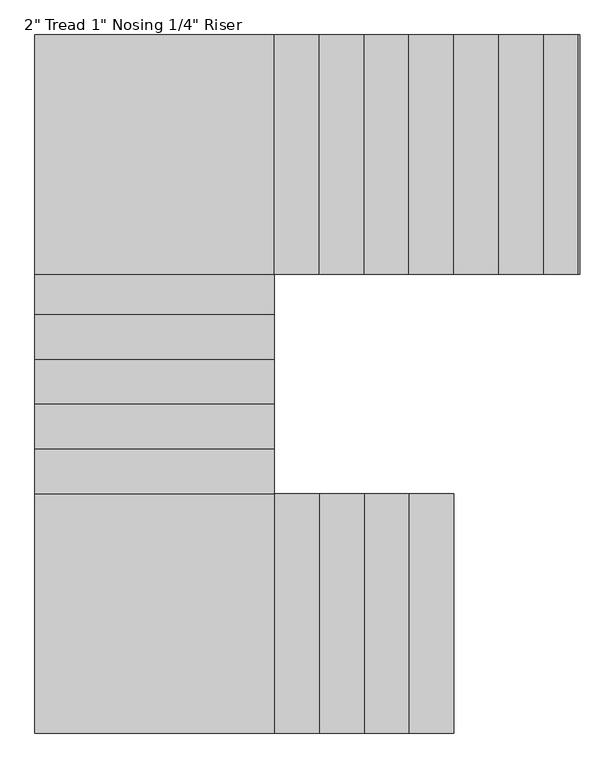
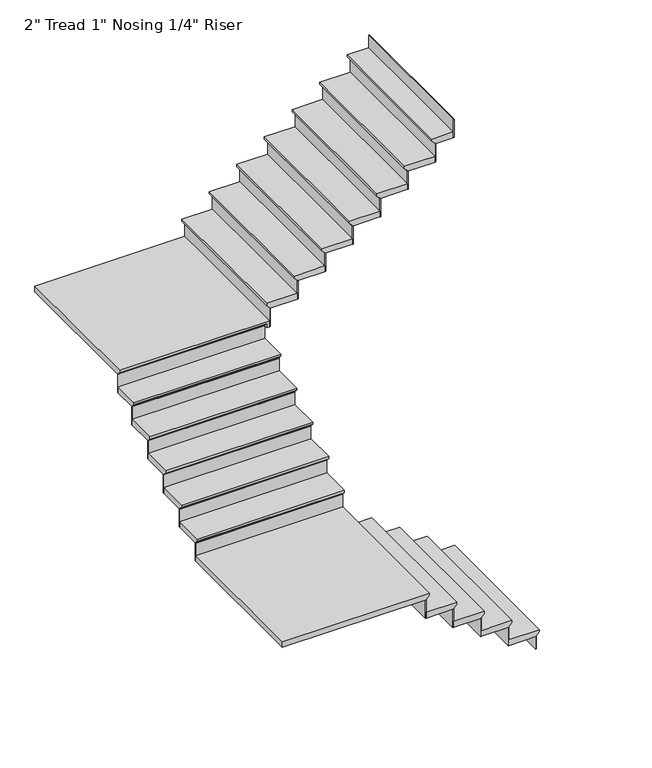
"""IFC4 building model written with IfcOpenShell, lengths in millimetres: stair flight geometry."""

from ifc_helpers import new_model, si_unit, origin, place, context, project, spatial, faceted_brep, source, transform, mapped, element, save


def stair_flight_abd4a925(model_context):
    return source(origin(), model_context, "Body", "Brep", [
        faceted_brep([(-2683.1105391, -1521.8373761, 9590.1710526), (-2683.1105391, -1521.8373761, 9609.2210526), (-2683.1105391, -2741.0373761, 9609.2210526), (-2683.1105391, -2741.0373761, 9590.1710526), (-2708.5105391, -1521.8373761, 9564.7710526), (-2708.5105391, -2741.0373761, 9564.7710526), (-2937.1105391, -1521.8373761, 9609.2210526), (-2937.1105391, -2741.0373761, 9609.2210526), (-2708.5105391, -2741.0373761, 9558.4210526), (-2937.1105391, -2741.0373761, 9558.4210526), (-2937.1105391, -1521.8373761, 9558.4210526), (-2708.5105391, -1521.8373761, 9558.4210526)], [[[0, 1, 2, 3]], [[4, 0, 3, 5]], [[2, 1, 6, 7]], [[8, 9, 10, 11]], [[2, 7, 9, 8, 5, 3]], [[8, 11, 4, 5]], [[6, 1, 0, 4, 11, 10]], [[7, 6, 10, 9]]]),
        faceted_brep([(-2708.5105391, -1521.8373761, 9558.4210526), (-2708.5105391, -1521.8373761, 9448.8), (-2714.8605391, -1521.8373761, 9448.8), (-2714.8605391, -1521.8373761, 9558.4210526), (-2708.5105391, -2741.0373761, 9558.4210526), (-2714.8605391, -2741.0373761, 9558.4210526), (-2714.8605391, -2741.0373761, 9448.8), (-2708.5105391, -2741.0373761, 9448.8)], [[[0, 1, 2, 3]], [[4, 5, 6, 7]], [[1, 0, 4, 7]], [[2, 1, 7, 6]], [[3, 2, 6, 5]], [[0, 3, 5, 4]]]),
        faceted_brep([(-2937.1105391, -1521.8373761, 9718.8421053), (-2937.1105391, -1521.8373761, 9558.4210526), (-2943.4605391, -1521.8373761, 9558.4210526), (-2943.4605391, -1521.8373761, 9718.8421053), (-2937.1105391, -2741.0373761, 9718.8421053), (-2943.4605391, -2741.0373761, 9718.8421053), (-2943.4605391, -2741.0373761, 9558.4210526), (-2937.1105391, -2741.0373761, 9558.4210526)], [[[0, 1, 2, 3]], [[4, 5, 6, 7]], [[1, 0, 4, 7]], [[2, 1, 7, 6]], [[3, 2, 6, 5]], [[0, 3, 5, 4]]]),
        faceted_brep([(-2911.7105391, -2741.0373761, 9769.6421053), (-2911.7105391, -1521.8373761, 9769.6421053), (-3165.7105391, -1521.8373761, 9769.6421053), (-3165.7105391, -2741.0373761, 9769.6421053), (-2937.1105391, -2741.0373761, 9718.8421053), (-3165.7105391, -2741.0373761, 9718.8421053), (-3165.7105391, -1521.8373761, 9718.8421053), (-2937.1105391, -1521.8373761, 9718.8421053), (-2937.1105391, -2741.0373761, 9725.1921053), (-2911.7105391, -2741.0373761, 9750.5921053), (-2937.1105391, -1521.8373761, 9725.1921053), (-2911.7105391, -1521.8373761, 9750.5921053)], [[[0, 1, 2, 3]], [[4, 5, 6, 7]], [[0, 3, 5, 4, 8, 9]], [[4, 7, 10, 8]], [[2, 1, 11, 10, 7, 6]], [[3, 2, 6, 5]], [[11, 1, 0, 9]], [[10, 11, 9, 8]]]),
        faceted_brep([(-3165.7105391, -1521.8373761, 9879.2631579), (-3165.7105391, -1521.8373761, 9718.8421053), (-3172.0605391, -1521.8373761, 9718.8421053), (-3172.0605391, -1521.8373761, 9879.2631579), (-3165.7105391, -2741.0373761, 9879.2631579), (-3172.0605391, -2741.0373761, 9879.2631579), (-3172.0605391, -2741.0373761, 9718.8421053), (-3165.7105391, -2741.0373761, 9718.8421053)], [[[0, 1, 2, 3]], [[4, 5, 6, 7]], [[1, 0, 4, 7]], [[2, 1, 7, 6]], [[3, 2, 6, 5]], [[0, 3, 5, 4]]]),
        faceted_brep([(-3140.3105391, -2741.0373761, 9930.0631579), (-3140.3105391, -1521.8373761, 9930.0631579), (-3394.3105391, -1521.8373761, 9930.0631579), (-3394.3105391, -2741.0373761, 9930.0631579), (-3165.7105391, -2741.0373761, 9879.2631579), (-3394.3105391, -2741.0373761, 9879.2631579), (-3394.3105391, -1521.8373761, 9879.2631579), (-3165.7105391, -1521.8373761, 9879.2631579), (-3165.7105391, -2741.0373761, 9885.6131579), (-3140.3105391, -2741.0373761, 9911.0131579), (-3165.7105391, -1521.8373761, 9885.6131579), (-3140.3105391, -1521.8373761, 9911.0131579)], [[[0, 1, 2, 3]], [[4, 5, 6, 7]], [[0, 3, 5, 4, 8, 9]], [[4, 7, 10, 8]], [[2, 1, 11, 10, 7, 6]], [[3, 2, 6, 5]], [[11, 1, 0, 9]], [[10, 11, 9, 8]]]),
        faceted_brep([(-3394.3105391, -1521.8373761, 10039.6842105), (-3394.3105391, -1521.8373761, 9879.2631579), (-3400.6605391, -1521.8373761, 9879.2631579), (-3400.6605391, -1521.8373761, 10039.6842105), (-3394.3105391, -2741.0373761, 10039.6842105), (-3400.6605391, -2741.0373761, 10039.6842105), (-3400.6605391, -2741.0373761, 9879.2631579), (-3394.3105391, -2741.0373761, 9879.2631579)], [[[0, 1, 2, 3]], [[4, 5, 6, 7]], [[1, 0, 4, 7]], [[2, 1, 7, 6]], [[3, 2, 6, 5]], [[0, 3, 5, 4]]]),
        faceted_brep([(-3368.9105391, -2741.0373761, 10090.4842105), (-3368.9105391, -1521.8373761, 10090.4842105), (-3622.9105391, -1521.8373761, 10090.4842105), (-3622.9105391, -2741.0373761, 10090.4842105), (-3394.3105391, -2741.0373761, 10039.6842105), (-3622.9105391, -2741.0373761, 10039.6842105), (-3622.9105391, -1521.8373761, 10039.6842105), (-3394.3105391, -1521.8373761, 10039.6842105), (-3394.3105391, -2741.0373761, 10046.0342105), (-3368.9105391, -2741.0373761, 10071.4342105), (-3394.3105391, -1521.8373761, 10046.0342105), (-3368.9105391, -1521.8373761, 10071.4342105)], [[[0, 1, 2, 3]], [[4, 5, 6, 7]], [[0, 3, 5, 4, 8, 9]], [[4, 7, 10, 8]], [[2, 1, 11, 10, 7, 6]], [[3, 2, 6, 5]], [[11, 1, 0, 9]], [[10, 11, 9, 8]]]),
        faceted_brep([(-3622.9105391, -1521.8373761, 10200.1052632), (-3622.9105391, -1521.8373761, 10039.6842105), (-3629.2605391, -1521.8373761, 10039.6842105), (-3629.2605391, -1521.8373761, 10200.1052632), (-3622.9105391, -2741.0373761, 10200.1052632), (-3629.2605391, -2741.0373761, 10200.1052632), (-3629.2605391, -2741.0373761, 10039.6842105), (-3622.9105391, -2741.0373761, 10039.6842105)], [[[0, 1, 2, 3]], [[4, 5, 6, 7]], [[1, 0, 4, 7]], [[2, 1, 7, 6]], [[3, 2, 6, 5]], [[0, 3, 5, 4]]]),
        faceted_brep([(-4816.7105391, -1496.4373761, 10250.9052632), (-4816.7105391, -2741.0373761, 10250.9052632), (-3597.5105391, -2741.0373761, 10250.9052632), (-3597.5105391, -1496.4373761, 10250.9052632), (-4816.7105391, -2741.0373761, 10200.1052632), (-4816.7105391, -1496.4373761, 10200.1052632), (-3597.5105391, -1496.4373761, 10200.1052632), (-3597.5105391, -1521.8373761, 10200.1052632), (-3622.9105391, -1521.8373761, 10200.1052632), (-3622.9105391, -2741.0373761, 10200.1052632), (-3622.9105391, -2741.0373761, 10206.4552632), (-3597.5105391, -2741.0373761, 10231.8552632), (-3622.9105391, -1521.8373761, 10206.4552632), (-3597.5105391, -1521.8373761, 10231.8552632)], [[[0, 1, 2, 3]], [[4, 5, 6, 7, 8, 9]], [[1, 0, 5, 4]], [[2, 1, 4, 9, 10, 11]], [[9, 8, 12, 10]], [[8, 7, 13, 12]], [[3, 2, 11, 13, 7, 6]], [[0, 3, 6, 5]], [[11, 10, 12, 13]]]),
        faceted_brep([(-3597.5105391, -1496.4373761, 10360.5263158), (-3597.5105391, -1496.4373761, 10200.1052632), (-3597.5105391, -1490.0873761, 10200.1052632), (-3597.5105391, -1490.0873761, 10360.5263158), (-4816.7105391, -1496.4373761, 10360.5263158), (-4816.7105391, -1490.0873761, 10360.5263158), (-4816.7105391, -1490.0873761, 10200.1052632), (-4816.7105391, -1496.4373761, 10200.1052632)], [[[0, 1, 2, 3]], [[4, 5, 6, 7]], [[1, 0, 4, 7]], [[2, 1, 7, 6]], [[3, 2, 6, 5]], [[0, 3, 5, 4]]]),
        faceted_brep([(-4816.7105391, -1521.8373761, 10411.3263158), (-3597.5105391, -1521.8373761, 10411.3263158), (-3597.5105391, -1267.8373761, 10411.3263158), (-4816.7105391, -1267.8373761, 10411.3263158), (-4816.7105391, -1496.4373761, 10360.5263158), (-4816.7105391, -1267.8373761, 10360.5263158), (-3597.5105391, -1267.8373761, 10360.5263158), (-3597.5105391, -1496.4373761, 10360.5263158), (-4816.7105391, -1496.4373761, 10366.8763158), (-4816.7105391, -1521.8373761, 10392.2763158), (-3597.5105391, -1496.4373761, 10366.8763158), (-3597.5105391, -1521.8373761, 10392.2763158)], [[[0, 1, 2, 3]], [[4, 5, 6, 7]], [[0, 3, 5, 4, 8, 9]], [[4, 7, 10, 8]], [[2, 1, 11, 10, 7, 6]], [[3, 2, 6, 5]], [[11, 1, 0, 9]], [[10, 11, 9, 8]]]),
        faceted_brep([(-3597.5105391, -1267.8373761, 10520.9473684), (-3597.5105391, -1267.8373761, 10360.5263158), (-3597.5105391, -1261.4873761, 10360.5263158), (-3597.5105391, -1261.4873761, 10520.9473684), (-4816.7105391, -1267.8373761, 10520.9473684), (-4816.7105391, -1261.4873761, 10520.9473684), (-4816.7105391, -1261.4873761, 10360.5263158), (-4816.7105391, -1267.8373761, 10360.5263158)], [[[0, 1, 2, 3]], [[4, 5, 6, 7]], [[1, 0, 4, 7]], [[2, 1, 7, 6]], [[3, 2, 6, 5]], [[0, 3, 5, 4]]]),
        faceted_brep([(-4816.7105391, -1293.2373761, 10571.7473684), (-3597.5105391, -1293.2373761, 10571.7473684), (-3597.5105391, -1039.2373761, 10571.7473684), (-4816.7105391, -1039.2373761, 10571.7473684), (-4816.7105391, -1267.8373761, 10520.9473684), (-4816.7105391, -1039.2373761, 10520.9473684), (-3597.5105391, -1039.2373761, 10520.9473684), (-3597.5105391, -1267.8373761, 10520.9473684), (-4816.7105391, -1267.8373761, 10527.2973684), (-4816.7105391, -1293.2373761, 10552.6973684), (-3597.5105391, -1267.8373761, 10527.2973684), (-3597.5105391, -1293.2373761, 10552.6973684)], [[[0, 1, 2, 3]], [[4, 5, 6, 7]], [[0, 3, 5, 4, 8, 9]], [[4, 7, 10, 8]], [[2, 1, 11, 10, 7, 6]], [[3, 2, 6, 5]], [[11, 1, 0, 9]], [[10, 11, 9, 8]]]),
        faceted_brep([(-3597.5105391, -1039.2373761, 10681.3684211), (-3597.5105391, -1039.2373761, 10520.9473684), (-3597.5105391, -1032.8873761, 10520.9473684), (-3597.5105391, -1032.8873761, 10681.3684211), (-4816.7105391, -1039.2373761, 10681.3684211), (-4816.7105391, -1032.8873761, 10681.3684211), (-4816.7105391, -1032.8873761, 10520.9473684), (-4816.7105391, -1039.2373761, 10520.9473684)], [[[0, 1, 2, 3]], [[4, 5, 6, 7]], [[1, 0, 4, 7]], [[2, 1, 7, 6]], [[3, 2, 6, 5]], [[0, 3, 5, 4]]]),
        faceted_brep([(-4816.7105391, -1064.6373761, 10732.1684211), (-3597.5105391, -1064.6373761, 10732.1684211), (-3597.5105391, -810.6373761, 10732.1684211), (-4816.7105391, -810.6373761, 10732.1684211), (-4816.7105391, -1039.2373761, 10681.3684211), (-4816.7105391, -810.6373761, 10681.3684211), (-3597.5105391, -810.6373761, 10681.3684211), (-3597.5105391, -1039.2373761, 10681.3684211), (-4816.7105391, -1039.2373761, 10687.7184211), (-4816.7105391, -1064.6373761, 10713.1184211), (-3597.5105391, -1039.2373761, 10687.7184211), (-3597.5105391, -1064.6373761, 10713.1184211)], [[[0, 1, 2, 3]], [[4, 5, 6, 7]], [[0, 3, 5, 4, 8, 9]], [[4, 7, 10, 8]], [[2, 1, 11, 10, 7, 6]], [[3, 2, 6, 5]], [[11, 1, 0, 9]], [[10, 11, 9, 8]]]),
        faceted_brep([(-3597.5105391, -810.6373761, 10841.7894737), (-3597.5105391, -810.6373761, 10681.3684211), (-3597.5105391, -804.2873761, 10681.3684211), (-3597.5105391, -804.2873761, 10841.7894737), (-4816.7105391, -810.6373761, 10841.7894737), (-4816.7105391, -804.2873761, 10841.7894737), (-4816.7105391, -804.2873761, 10681.3684211), (-4816.7105391, -810.6373761, 10681.3684211)], [[[0, 1, 2, 3]], [[4, 5, 6, 7]], [[1, 0, 4, 7]], [[2, 1, 7, 6]], [[3, 2, 6, 5]], [[0, 3, 5, 4]]]),
        faceted_brep([(-4816.7105391, -836.0373761, 10892.5894737), (-3597.5105391, -836.0373761, 10892.5894737), (-3597.5105391, -582.0373761, 10892.5894737), (-4816.7105391, -582.0373761, 10892.5894737), (-4816.7105391, -810.6373761, 10841.7894737), (-4816.7105391, -582.0373761, 10841.7894737), (-3597.5105391, -582.0373761, 10841.7894737), (-3597.5105391, -810.6373761, 10841.7894737), (-4816.7105391, -810.6373761, 10848.1394737), (-4816.7105391, -836.0373761, 10873.5394737), (-3597.5105391, -810.6373761, 10848.1394737), (-3597.5105391, -836.0373761, 10873.5394737)], [[[0, 1, 2, 3]], [[4, 5, 6, 7]], [[0, 3, 5, 4, 8, 9]], [[4, 7, 10, 8]], [[2, 1, 11, 10, 7, 6]], [[3, 2, 6, 5]], [[11, 1, 0, 9]], [[10, 11, 9, 8]]]),
        faceted_brep([(-3597.5105391, -582.0373761, 11002.2105263), (-3597.5105391, -582.0373761, 10841.7894737), (-3597.5105391, -575.6873761, 10841.7894737), (-3597.5105391, -575.6873761, 11002.2105263), (-4816.7105391, -582.0373761, 11002.2105263), (-4816.7105391, -575.6873761, 11002.2105263), (-4816.7105391, -575.6873761, 10841.7894737), (-4816.7105391, -582.0373761, 10841.7894737)], [[[0, 1, 2, 3]], [[4, 5, 6, 7]], [[1, 0, 4, 7]], [[2, 1, 7, 6]], [[3, 2, 6, 5]], [[0, 3, 5, 4]]]),
        faceted_brep([(-4816.7105391, -607.4373761, 11053.0105263), (-3597.5105391, -607.4373761, 11053.0105263), (-3597.5105391, -378.8373761, 11053.0105263), (-4816.7105391, -378.8373761, 11053.0105263), (-4816.7105391, -582.0373761, 11002.2105263), (-4816.7105391, -378.8373761, 11002.2105263), (-3597.5105391, -378.8373761, 11002.2105263), (-3597.5105391, -582.0373761, 11002.2105263), (-4816.7105391, -582.0373761, 11008.5605263), (-4816.7105391, -607.4373761, 11033.9605263), (-3597.5105391, -582.0373761, 11008.5605263), (-3597.5105391, -607.4373761, 11033.9605263)], [[[0, 1, 2, 3]], [[4, 5, 6, 7]], [[0, 3, 5, 4, 8, 9]], [[4, 7, 10, 8]], [[2, 1, 11, 10, 7, 6]], [[3, 2, 6, 5]], [[11, 1, 0, 9]], [[10, 11, 9, 8]]]),
        faceted_brep([(-3597.5105391, -378.8373761, 11162.6315789), (-3597.5105391, -378.8373761, 11002.2105263), (-3597.5105391, -372.4873761, 11002.2105263), (-3597.5105391, -372.4873761, 11162.6315789), (-4816.7105391, -378.8373761, 11162.6315789), (-4816.7105391, -372.4873761, 11162.6315789), (-4816.7105391, -372.4873761, 11002.2105263), (-4816.7105391, -378.8373761, 11002.2105263)], [[[0, 1, 2, 3]], [[4, 5, 6, 7]], [[1, 0, 4, 7]], [[2, 1, 7, 6]], [[3, 2, 6, 5]], [[0, 3, 5, 4]]]),
        faceted_brep([(-3572.1105391, 814.9626239, 11213.4315789), (-4816.7105391, 814.9626239, 11213.4315789), (-4816.7105391, -404.2373761, 11213.4315789), (-3572.1105391, -404.2373761, 11213.4315789), (-4816.7105391, 814.9626239, 11162.6315789), (-3572.1105391, 814.9626239, 11162.6315789), (-3572.1105391, -404.2373761, 11162.6315789), (-3597.5105391, -404.2373761, 11162.6315789), (-3597.5105391, -378.8373761, 11162.6315789), (-4816.7105391, -378.8373761, 11162.6315789), (-4816.7105391, -378.8373761, 11168.9815789), (-4816.7105391, -404.2373761, 11194.3815789), (-3597.5105391, -378.8373761, 11168.9815789), (-3597.5105391, -404.2373761, 11194.3815789)], [[[0, 1, 2, 3]], [[4, 5, 6, 7, 8, 9]], [[1, 0, 5, 4]], [[2, 1, 4, 9, 10, 11]], [[9, 8, 12, 10]], [[8, 7, 13, 12]], [[3, 2, 11, 13, 7, 6]], [[0, 3, 6, 5]], [[11, 10, 12, 13]]]),
        faceted_brep([(-3572.1105391, -404.2373761, 11323.0526316), (-3572.1105391, -404.2373761, 11162.6315789), (-3565.7605391, -404.2373761, 11162.6315789), (-3565.7605391, -404.2373761, 11323.0526316), (-3572.1105391, 814.9626239, 11323.0526316), (-3565.7605391, 814.9626239, 11323.0526316), (-3565.7605391, 814.9626239, 11162.6315789), (-3572.1105391, 814.9626239, 11162.6315789)], [[[0, 1, 2, 3]], [[4, 5, 6, 7]], [[1, 0, 4, 7]], [[2, 1, 7, 6]], [[3, 2, 6, 5]], [[0, 3, 5, 4]]]),
        faceted_brep([(-3597.5105391, 814.9626239, 11373.8526316), (-3597.5105391, -404.2373761, 11373.8526316), (-3343.5105391, -404.2373761, 11373.8526316), (-3343.5105391, 814.9626239, 11373.8526316), (-3572.1105391, 814.9626239, 11323.0526316), (-3343.5105391, 814.9626239, 11323.0526316), (-3343.5105391, -404.2373761, 11323.0526316), (-3572.1105391, -404.2373761, 11323.0526316), (-3572.1105391, 814.9626239, 11329.4026316), (-3597.5105391, 814.9626239, 11354.8026316), (-3572.1105391, -404.2373761, 11329.4026316), (-3597.5105391, -404.2373761, 11354.8026316)], [[[0, 1, 2, 3]], [[4, 5, 6, 7]], [[0, 3, 5, 4, 8, 9]], [[4, 7, 10, 8]], [[2, 1, 11, 10, 7, 6]], [[3, 2, 6, 5]], [[11, 1, 0, 9]], [[10, 11, 9, 8]]]),
        faceted_brep([(-3343.5105391, -404.2373761, 11483.4736842), (-3343.5105391, -404.2373761, 11323.0526316), (-3337.1605391, -404.2373761, 11323.0526316), (-3337.1605391, -404.2373761, 11483.4736842), (-3343.5105391, 814.9626239, 11483.4736842), (-3337.1605391, 814.9626239, 11483.4736842), (-3337.1605391, 814.9626239, 11323.0526316), (-3343.5105391, 814.9626239, 11323.0526316)], [[[0, 1, 2, 3]], [[4, 5, 6, 7]], [[1, 0, 4, 7]], [[2, 1, 7, 6]], [[3, 2, 6, 5]], [[0, 3, 5, 4]]]),
        faceted_brep([(-3368.9105391, 814.9626239, 11534.2736842), (-3368.9105391, -404.2373761, 11534.2736842), (-3114.9105391, -404.2373761, 11534.2736842), (-3114.9105391, 814.9626239, 11534.2736842), (-3343.5105391, 814.9626239, 11483.4736842), (-3114.9105391, 814.9626239, 11483.4736842), (-3114.9105391, -404.2373761, 11483.4736842), (-3343.5105391, -404.2373761, 11483.4736842), (-3343.5105391, 814.9626239, 11489.8236842), (-3368.9105391, 814.9626239, 11515.2236842), (-3343.5105391, -404.2373761, 11489.8236842), (-3368.9105391, -404.2373761, 11515.2236842)], [[[0, 1, 2, 3]], [[4, 5, 6, 7]], [[0, 3, 5, 4, 8, 9]], [[4, 7, 10, 8]], [[2, 1, 11, 10, 7, 6]], [[3, 2, 6, 5]], [[11, 1, 0, 9]], [[10, 11, 9, 8]]]),
        faceted_brep([(-3114.9105391, -404.2373761, 11643.8947368), (-3114.9105391, -404.2373761, 11483.4736842), (-3108.5605391, -404.2373761, 11483.4736842), (-3108.5605391, -404.2373761, 11643.8947368), (-3114.9105391, 814.9626239, 11643.8947368), (-3108.5605391, 814.9626239, 11643.8947368), (-3108.5605391, 814.9626239, 11483.4736842), (-3114.9105391, 814.9626239, 11483.4736842)], [[[0, 1, 2, 3]], [[4, 5, 6, 7]], [[1, 0, 4, 7]], [[2, 1, 7, 6]], [[3, 2, 6, 5]], [[0, 3, 5, 4]]]),
        faceted_brep([(-3140.3105391, 814.9626239, 11694.6947368), (-3140.3105391, -404.2373761, 11694.6947368), (-2886.3105391, -404.2373761, 11694.6947368), (-2886.3105391, 814.9626239, 11694.6947368), (-3114.9105391, 814.9626239, 11643.8947368), (-2886.3105391, 814.9626239, 11643.8947368), (-2886.3105391, -404.2373761, 11643.8947368), (-3114.9105391, -404.2373761, 11643.8947368), (-3114.9105391, 814.9626239, 11650.2447368), (-3140.3105391, 814.9626239, 11675.6447368), (-3114.9105391, -404.2373761, 11650.2447368), (-3140.3105391, -404.2373761, 11675.6447368)], [[[0, 1, 2, 3]], [[4, 5, 6, 7]], [[0, 3, 5, 4, 8, 9]], [[4, 7, 10, 8]], [[2, 1, 11, 10, 7, 6]], [[3, 2, 6, 5]], [[11, 1, 0, 9]], [[10, 11, 9, 8]]]),
        faceted_brep([(-2886.3105391, -404.2373761, 11804.3157895), (-2886.3105391, -404.2373761, 11643.8947368), (-2879.9605391, -404.2373761, 11643.8947368), (-2879.9605391, -404.2373761, 11804.3157895), (-2886.3105391, 814.9626239, 11804.3157895), (-2879.9605391, 814.9626239, 11804.3157895), (-2879.9605391, 814.9626239, 11643.8947368), (-2886.3105391, 814.9626239, 11643.8947368)], [[[0, 1, 2, 3]], [[4, 5, 6, 7]], [[1, 0, 4, 7]], [[2, 1, 7, 6]], [[3, 2, 6, 5]], [[0, 3, 5, 4]]]),
        faceted_brep([(-2911.7105391, 814.9626239, 11855.1157895), (-2911.7105391, -404.2373761, 11855.1157895), (-2657.7105391, -404.2373761, 11855.1157895), (-2657.7105391, 814.9626239, 11855.1157895), (-2886.3105391, 814.9626239, 11804.3157895), (-2657.7105391, 814.9626239, 11804.3157895), (-2657.7105391, -404.2373761, 11804.3157895), (-2886.3105391, -404.2373761, 11804.3157895), (-2886.3105391, 814.9626239, 11810.6657895), (-2911.7105391, 814.9626239, 11836.0657895), (-2886.3105391, -404.2373761, 11810.6657895), (-2911.7105391, -404.2373761, 11836.0657895)], [[[0, 1, 2, 3]], [[4, 5, 6, 7]], [[0, 3, 5, 4, 8, 9]], [[4, 7, 10, 8]], [[2, 1, 11, 10, 7, 6]], [[3, 2, 6, 5]], [[11, 1, 0, 9]], [[10, 11, 9, 8]]]),
        faceted_brep([(-2657.7105391, -404.2373761, 11964.7368421), (-2657.7105391, -404.2373761, 11804.3157895), (-2651.3605391, -404.2373761, 11804.3157895), (-2651.3605391, -404.2373761, 11964.7368421), (-2657.7105391, 814.9626239, 11964.7368421), (-2651.3605391, 814.9626239, 11964.7368421), (-2651.3605391, 814.9626239, 11804.3157895), (-2657.7105391, 814.9626239, 11804.3157895)], [[[0, 1, 2, 3]], [[4, 5, 6, 7]], [[1, 0, 4, 7]], [[2, 1, 7, 6]], [[3, 2, 6, 5]], [[0, 3, 5, 4]]]),
        faceted_brep([(-2683.1105391, 814.9626239, 12015.5368421), (-2683.1105391, -404.2373761, 12015.5368421), (-2429.1105391, -404.2373761, 12015.5368421), (-2429.1105391, 814.9626239, 12015.5368421), (-2657.7105391, 814.9626239, 11964.7368421), (-2429.1105391, 814.9626239, 11964.7368421), (-2429.1105391, -404.2373761, 11964.7368421), (-2657.7105391, -404.2373761, 11964.7368421), (-2657.7105391, 814.9626239, 11971.0868421), (-2683.1105391, 814.9626239, 11996.4868421), (-2657.7105391, -404.2373761, 11971.0868421), (-2683.1105391, -404.2373761, 11996.4868421)], [[[0, 1, 2, 3]], [[4, 5, 6, 7]], [[0, 3, 5, 4, 8, 9]], [[4, 7, 10, 8]], [[2, 1, 11, 10, 7, 6]], [[3, 2, 6, 5]], [[11, 1, 0, 9]], [[10, 11, 9, 8]]]),
        faceted_brep([(-2429.1105391, -404.2373761, 12125.1578947), (-2429.1105391, -404.2373761, 11964.7368421), (-2422.7605391, -404.2373761, 11964.7368421), (-2422.7605391, -404.2373761, 12125.1578947), (-2429.1105391, 814.9626239, 12125.1578947), (-2422.7605391, 814.9626239, 12125.1578947), (-2422.7605391, 814.9626239, 11964.7368421), (-2429.1105391, 814.9626239, 11964.7368421)], [[[0, 1, 2, 3]], [[4, 5, 6, 7]], [[1, 0, 4, 7]], [[2, 1, 7, 6]], [[3, 2, 6, 5]], [[0, 3, 5, 4]]]),
        faceted_brep([(-2454.5105391, 814.9626239, 12175.9578947), (-2454.5105391, -404.2373761, 12175.9578947), (-2200.5105391, -404.2373761, 12175.9578947), (-2200.5105391, 814.9626239, 12175.9578947), (-2429.1105391, 814.9626239, 12125.1578947), (-2200.5105391, 814.9626239, 12125.1578947), (-2200.5105391, -404.2373761, 12125.1578947), (-2429.1105391, -404.2373761, 12125.1578947), (-2429.1105391, 814.9626239, 12131.5078947), (-2454.5105391, 814.9626239, 12156.9078947), (-2429.1105391, -404.2373761, 12131.5078947), (-2454.5105391, -404.2373761, 12156.9078947)], [[[0, 1, 2, 3]], [[4, 5, 6, 7]], [[0, 3, 5, 4, 8, 9]], [[4, 7, 10, 8]], [[2, 1, 11, 10, 7, 6]], [[3, 2, 6, 5]], [[11, 1, 0, 9]], [[10, 11, 9, 8]]]),
        faceted_brep([(-2200.5105391, -404.2373761, 12285.5789474), (-2200.5105391, -404.2373761, 12125.1578947), (-2194.1605391, -404.2373761, 12125.1578947), (-2194.1605391, -404.2373761, 12285.5789474), (-2200.5105391, 814.9626239, 12285.5789474), (-2194.1605391, 814.9626239, 12285.5789474), (-2194.1605391, 814.9626239, 12125.1578947), (-2200.5105391, 814.9626239, 12125.1578947)], [[[0, 1, 2, 3]], [[4, 5, 6, 7]], [[1, 0, 4, 7]], [[2, 1, 7, 6]], [[3, 2, 6, 5]], [[0, 3, 5, 4]]]),
        faceted_brep([(-2048.1105391, -404.2373761, 12446.0), (-2048.1105391, -404.2373761, 12285.5789474), (-2041.7605391, -404.2373761, 12285.5789474), (-2041.7605391, -404.2373761, 12446.0), (-2048.1105391, 814.9626239, 12446.0), (-2041.7605391, 814.9626239, 12446.0), (-2041.7605391, 814.9626239, 12285.5789474), (-2048.1105391, 814.9626239, 12285.5789474)], [[[0, 1, 2, 3]], [[4, 5, 6, 7]], [[1, 0, 4, 7]], [[2, 1, 7, 6]], [[3, 2, 6, 5]], [[0, 3, 5, 4]]]),
        faceted_brep([(-2225.9105391, 814.9626239, 12336.3789474), (-2225.9105391, -404.2373761, 12336.3789474), (-2048.1105391, -404.2373761, 12336.3789474), (-2048.1105391, 814.9626239, 12336.3789474), (-2200.5105391, 814.9626239, 12285.5789474), (-2048.1105391, 814.9626239, 12285.5789474), (-2048.1105391, -404.2373761, 12285.5789474), (-2200.5105391, -404.2373761, 12285.5789474), (-2200.5105391, 814.9626239, 12291.9289474), (-2225.9105391, 814.9626239, 12317.3289474), (-2200.5105391, -404.2373761, 12291.9289474), (-2225.9105391, -404.2373761, 12317.3289474)], [[[0, 1, 2, 3]], [[4, 5, 6, 7]], [[0, 3, 5, 4, 8, 9]], [[4, 7, 10, 8]], [[2, 1, 11, 10, 7, 6]], [[3, 2, 6, 5]], [[11, 1, 0, 9]], [[10, 11, 9, 8]]]),
    ])


if __name__ == "__main__":
    model = new_model("IFC4")
    model_context = context("Model", 3, world=origin())
    ifc_project = project(units=[si_unit("LENGTHUNIT", "METRE", prefix="MILLI")], contexts=[model_context])
    site = spatial("IfcSite", under=ifc_project)
    building = spatial("IfcBuilding", under=site)
    placement = place(None, origin())
    stair_flight_shape = stair_flight_abd4a925(model_context)
    element("IfcStairFlight", 1, ObjectType="2\" Tread 1\" Nosing 1/4\" Riser", at=placement, inside=building, context=model_context, shape_type="MappedRepresentation", body=[
        mapped(stair_flight_shape, transform((0.0, 0.0, 0.0), x_axis=(1.0, 0.0, 0.0), y_axis=(0.0, 1.0, 0.0), z_axis=(0.0, 0.0, 1.0))),
    ])
    save(model, "model.ifc")
